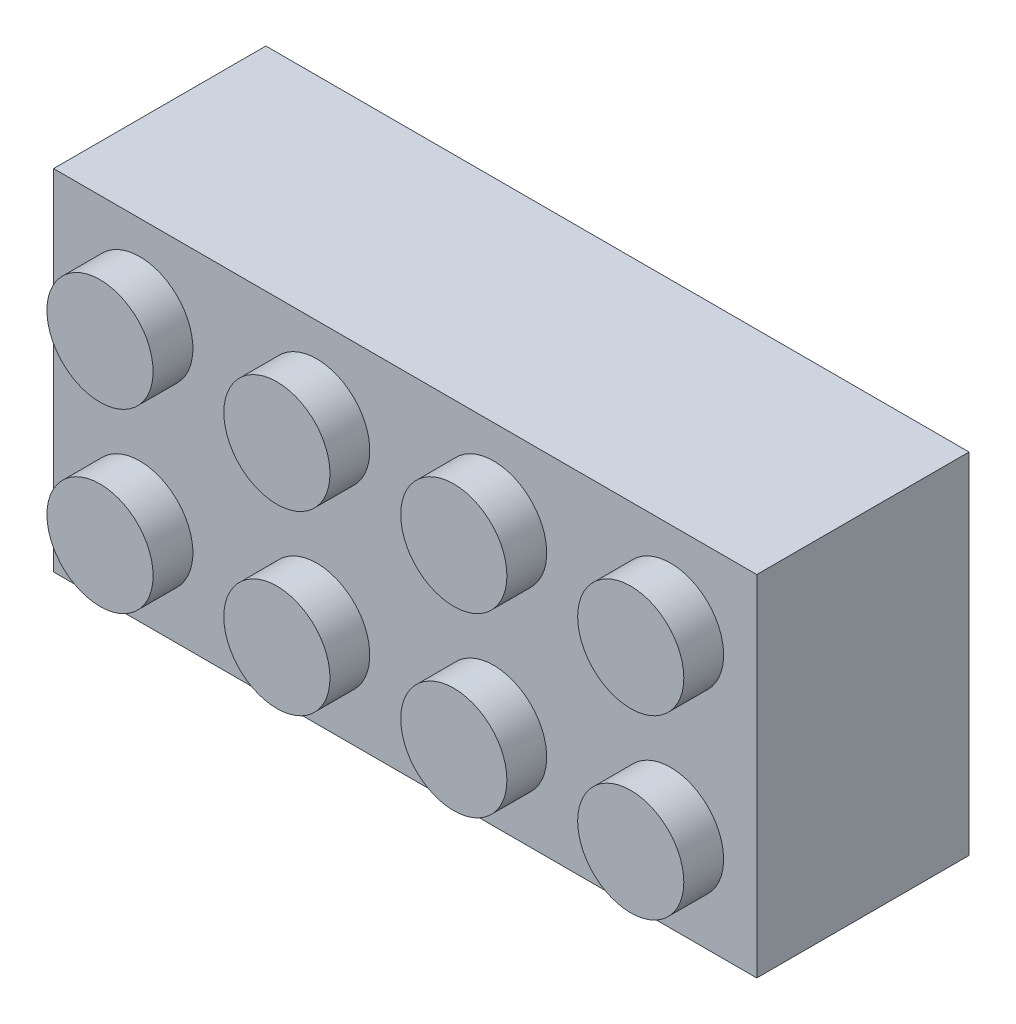
ISO-10303-21;
HEADER;
FILE_DESCRIPTION(('STEP AP214'),'2;1');
FILE_NAME('part.step','',(''),(''),'','','');
FILE_SCHEMA(('AUTOMOTIVE_DESIGN { 1 0 10303 214 1 1 1 1 }'));
ENDSEC;
DATA;
#1=APPLICATION_CONTEXT('core data for automotive mechanical design processes');
#2=APPLICATION_PROTOCOL_DEFINITION('international standard','automotive_design',2000,#1);
#3=PRODUCT_CONTEXT('',#1,'mechanical');
#4=PRODUCT('Part','Part','',(#3));
#5=PRODUCT_RELATED_PRODUCT_CATEGORY('part','',(#4));
#6=PRODUCT_DEFINITION_FORMATION('','',#4);
#7=PRODUCT_DEFINITION_CONTEXT('part definition',#1,'design');
#8=PRODUCT_DEFINITION('design','',#6,#7);
#9=PRODUCT_DEFINITION_SHAPE('','',#8);
#10=(LENGTH_UNIT() NAMED_UNIT(*) SI_UNIT(.MILLI.,.METRE.));
#11=(NAMED_UNIT(*) PLANE_ANGLE_UNIT() SI_UNIT($,.RADIAN.));
#12=(NAMED_UNIT(*) SI_UNIT($,.STERADIAN.) SOLID_ANGLE_UNIT());
#13=UNCERTAINTY_MEASURE_WITH_UNIT(LENGTH_MEASURE(1.E-05),#10,'distance_accuracy_value','');
#14=(GEOMETRIC_REPRESENTATION_CONTEXT(3) GLOBAL_UNCERTAINTY_ASSIGNED_CONTEXT((#13)) GLOBAL_UNIT_ASSIGNED_CONTEXT((#10,
#11,#12)) REPRESENTATION_CONTEXT('',''));
#15=CARTESIAN_POINT('',(0.,0.,0.));
#16=DIRECTION('',(0.,0.,1.));
#17=DIRECTION('',(1.,0.,0.));
#18=AXIS2_PLACEMENT_3D('',#15,#16,#17);
#19=CARTESIAN_POINT('',(31.8,0.,9.6));
#20=DIRECTION('',(0.,1.,0.));
#21=DIRECTION('',(0.,0.,1.));
#22=AXIS2_PLACEMENT_3D('',#19,#20,#21);
#23=PLANE('',#22);
#24=DIRECTION('',(1.,0.,0.));
#25=VECTOR('',#24,1.);
#26=CARTESIAN_POINT('',(31.8,0.,0.));
#27=LINE('',#26,#25);
#28=CARTESIAN_POINT('',(0.,0.,0.));
#29=VERTEX_POINT('',#28);
#30=CARTESIAN_POINT('',(31.8,0.,0.));
#31=VERTEX_POINT('',#30);
#32=EDGE_CURVE('E186',#29,#31,#27,.T.);
#33=ORIENTED_EDGE('',*,*,#32,.T.);
#34=DIRECTION('',(0.,0.,-1.));
#35=VECTOR('',#34,1.);
#36=CARTESIAN_POINT('',(31.8,0.,9.6));
#37=LINE('',#36,#35);
#38=CARTESIAN_POINT('',(31.8,0.,9.6));
#39=VERTEX_POINT('',#38);
#40=EDGE_CURVE('E213',#39,#31,#37,.T.);
#41=ORIENTED_EDGE('',*,*,#40,.F.);
#42=DIRECTION('',(1.,0.,0.));
#43=VECTOR('',#42,1.);
#44=CARTESIAN_POINT('',(31.8,0.,9.6));
#45=LINE('',#44,#43);
#46=CARTESIAN_POINT('',(0.,0.,9.6));
#47=VERTEX_POINT('',#46);
#48=EDGE_CURVE('E190',#47,#39,#45,.T.);
#49=ORIENTED_EDGE('',*,*,#48,.F.);
#50=DIRECTION('',(0.,0.,-1.));
#51=VECTOR('',#50,1.);
#52=CARTESIAN_POINT('',(0.,0.,9.6));
#53=LINE('',#52,#51);
#54=EDGE_CURVE('E197',#47,#29,#53,.T.);
#55=ORIENTED_EDGE('',*,*,#54,.T.);
#56=EDGE_LOOP('',(#33,#41,#49,#55));
#57=FACE_BOUND('',#56,.T.);
#58=ADVANCED_FACE('F42',(#57),#23,.F.);
#59=CARTESIAN_POINT('',(31.8,15.8,9.6));
#60=DIRECTION('',(-1.,0.,0.));
#61=DIRECTION('',(0.,0.,1.));
#62=AXIS2_PLACEMENT_3D('',#59,#60,#61);
#63=PLANE('',#62);
#64=DIRECTION('',(0.,1.,0.));
#65=VECTOR('',#64,1.);
#66=CARTESIAN_POINT('',(31.8,15.8,0.));
#67=LINE('',#66,#65);
#68=CARTESIAN_POINT('',(31.8,15.8,0.));
#69=VERTEX_POINT('',#68);
#70=EDGE_CURVE('E199',#31,#69,#67,.T.);
#71=ORIENTED_EDGE('',*,*,#70,.T.);
#72=DIRECTION('',(0.,0.,-1.));
#73=VECTOR('',#72,1.);
#74=CARTESIAN_POINT('',(31.8,15.8,9.6));
#75=LINE('',#74,#73);
#76=CARTESIAN_POINT('',(31.8,15.8,9.6));
#77=VERTEX_POINT('',#76);
#78=EDGE_CURVE('E209',#77,#69,#75,.T.);
#79=ORIENTED_EDGE('',*,*,#78,.F.);
#80=DIRECTION('',(0.,1.,0.));
#81=VECTOR('',#80,1.);
#82=CARTESIAN_POINT('',(31.8,15.8,9.6));
#83=LINE('',#82,#81);
#84=EDGE_CURVE('E189',#39,#77,#83,.T.);
#85=ORIENTED_EDGE('',*,*,#84,.F.);
#86=ORIENTED_EDGE('',*,*,#40,.T.);
#87=EDGE_LOOP('',(#71,#79,#85,#86));
#88=FACE_BOUND('',#87,.T.);
#89=ADVANCED_FACE('F264',(#88),#63,.F.);
#90=CARTESIAN_POINT('',(0.,15.8,9.6));
#91=DIRECTION('',(0.,-1.,0.));
#92=DIRECTION('',(0.,0.,-1.));
#93=AXIS2_PLACEMENT_3D('',#90,#91,#92);
#94=PLANE('',#93);
#95=DIRECTION('',(-1.,0.,0.));
#96=VECTOR('',#95,1.);
#97=CARTESIAN_POINT('',(0.,15.8,0.));
#98=LINE('',#97,#96);
#99=CARTESIAN_POINT('',(0.,15.8,0.));
#100=VERTEX_POINT('',#99);
#101=EDGE_CURVE('E205',#69,#100,#98,.T.);
#102=ORIENTED_EDGE('',*,*,#101,.T.);
#103=DIRECTION('',(0.,0.,-1.));
#104=VECTOR('',#103,1.);
#105=CARTESIAN_POINT('',(0.,15.8,9.6));
#106=LINE('',#105,#104);
#107=CARTESIAN_POINT('',(0.,15.8,9.6));
#108=VERTEX_POINT('',#107);
#109=EDGE_CURVE('E210',#108,#100,#106,.T.);
#110=ORIENTED_EDGE('',*,*,#109,.F.);
#111=DIRECTION('',(-1.,0.,0.));
#112=VECTOR('',#111,1.);
#113=CARTESIAN_POINT('',(0.,15.8,9.6));
#114=LINE('',#113,#112);
#115=EDGE_CURVE('E195',#77,#108,#114,.T.);
#116=ORIENTED_EDGE('',*,*,#115,.F.);
#117=ORIENTED_EDGE('',*,*,#78,.T.);
#118=EDGE_LOOP('',(#102,#110,#116,#117));
#119=FACE_BOUND('',#118,.T.);
#120=ADVANCED_FACE('F269',(#119),#94,.F.);
#121=CARTESIAN_POINT('',(0.,0.,9.6));
#122=DIRECTION('',(1.,0.,0.));
#123=DIRECTION('',(0.,0.,-1.));
#124=AXIS2_PLACEMENT_3D('',#121,#122,#123);
#125=PLANE('',#124);
#126=DIRECTION('',(0.,-1.,0.));
#127=VECTOR('',#126,1.);
#128=CARTESIAN_POINT('',(0.,0.,0.));
#129=LINE('',#128,#127);
#130=EDGE_CURVE('E192',#100,#29,#129,.T.);
#131=ORIENTED_EDGE('',*,*,#130,.T.);
#132=ORIENTED_EDGE('',*,*,#54,.F.);
#133=DIRECTION('',(0.,-1.,0.));
#134=VECTOR('',#133,1.);
#135=CARTESIAN_POINT('',(0.,0.,9.6));
#136=LINE('',#135,#134);
#137=EDGE_CURVE('E193',#108,#47,#136,.T.);
#138=ORIENTED_EDGE('',*,*,#137,.F.);
#139=ORIENTED_EDGE('',*,*,#109,.T.);
#140=EDGE_LOOP('',(#131,#132,#138,#139));
#141=FACE_BOUND('',#140,.T.);
#142=ADVANCED_FACE('F245',(#141),#125,.F.);
#143=CARTESIAN_POINT('',(0.,0.,9.6));
#144=DIRECTION('',(0.,0.,-1.));
#145=DIRECTION('',(-1.,0.,0.));
#146=AXIS2_PLACEMENT_3D('',#143,#144,#145);
#147=PLANE('',#146);
#148=CARTESIAN_POINT('',(27.9,3.9,9.6));
#149=DIRECTION('',(0.,0.,-1.));
#150=DIRECTION('',(-1.,0.,0.));
#151=AXIS2_PLACEMENT_3D('',#148,#149,#150);
#152=CIRCLE('',#151,2.4);
#153=CARTESIAN_POINT('',(25.5,3.9,9.6));
#154=VERTEX_POINT('',#153);
#155=EDGE_CURVE('E11',#154,#154,#152,.F.);
#156=ORIENTED_EDGE('',*,*,#155,.F.);
#157=EDGE_LOOP('',(#156));
#158=FACE_BOUND('',#157,.T.);
#159=CARTESIAN_POINT('',(19.9,3.9,9.6));
#160=DIRECTION('',(0.,0.,-1.));
#161=DIRECTION('',(-1.,0.,0.));
#162=AXIS2_PLACEMENT_3D('',#159,#160,#161);
#163=CIRCLE('',#162,2.4);
#164=CARTESIAN_POINT('',(17.5,3.9,9.6));
#165=VERTEX_POINT('',#164);
#166=EDGE_CURVE('E55',#165,#165,#163,.F.);
#167=ORIENTED_EDGE('',*,*,#166,.F.);
#168=EDGE_LOOP('',(#167));
#169=FACE_BOUND('',#168,.T.);
#170=CARTESIAN_POINT('',(11.9,3.9,9.6));
#171=DIRECTION('',(0.,0.,-1.));
#172=DIRECTION('',(-1.,0.,0.));
#173=AXIS2_PLACEMENT_3D('',#170,#171,#172);
#174=CIRCLE('',#173,2.4);
#175=CARTESIAN_POINT('',(9.5,3.9,9.6));
#176=VERTEX_POINT('',#175);
#177=EDGE_CURVE('E232',#176,#176,#174,.F.);
#178=ORIENTED_EDGE('',*,*,#177,.F.);
#179=EDGE_LOOP('',(#178));
#180=FACE_BOUND('',#179,.T.);
#181=CARTESIAN_POINT('',(27.9,11.9,9.6));
#182=DIRECTION('',(0.,0.,-1.));
#183=DIRECTION('',(-1.,0.,0.));
#184=AXIS2_PLACEMENT_3D('',#181,#182,#183);
#185=CIRCLE('',#184,2.4);
#186=CARTESIAN_POINT('',(25.5,11.9,9.6));
#187=VERTEX_POINT('',#186);
#188=EDGE_CURVE('E227',#187,#187,#185,.F.);
#189=ORIENTED_EDGE('',*,*,#188,.F.);
#190=EDGE_LOOP('',(#189));
#191=FACE_BOUND('',#190,.T.);
#192=CARTESIAN_POINT('',(19.9,11.9,9.6));
#193=DIRECTION('',(0.,0.,-1.));
#194=DIRECTION('',(-1.,0.,0.));
#195=AXIS2_PLACEMENT_3D('',#192,#193,#194);
#196=CIRCLE('',#195,2.4);
#197=CARTESIAN_POINT('',(17.5,11.9,9.6));
#198=VERTEX_POINT('',#197);
#199=EDGE_CURVE('E223',#198,#198,#196,.F.);
#200=ORIENTED_EDGE('',*,*,#199,.F.);
#201=EDGE_LOOP('',(#200));
#202=FACE_BOUND('',#201,.T.);
#203=CARTESIAN_POINT('',(11.9,11.9,9.6));
#204=DIRECTION('',(0.,0.,-1.));
#205=DIRECTION('',(-1.,0.,0.));
#206=AXIS2_PLACEMENT_3D('',#203,#204,#205);
#207=CIRCLE('',#206,2.4);
#208=CARTESIAN_POINT('',(9.5,11.9,9.6));
#209=VERTEX_POINT('',#208);
#210=EDGE_CURVE('E225',#209,#209,#207,.F.);
#211=ORIENTED_EDGE('',*,*,#210,.F.);
#212=EDGE_LOOP('',(#211));
#213=FACE_BOUND('',#212,.T.);
#214=CARTESIAN_POINT('',(3.9,3.9,9.6));
#215=DIRECTION('',(0.,0.,-1.));
#216=DIRECTION('',(-1.,0.,0.));
#217=AXIS2_PLACEMENT_3D('',#214,#215,#216);
#218=CIRCLE('',#217,2.4);
#219=CARTESIAN_POINT('',(1.5,3.9,9.6));
#220=VERTEX_POINT('',#219);
#221=EDGE_CURVE('E218',#220,#220,#218,.F.);
#222=ORIENTED_EDGE('',*,*,#221,.F.);
#223=EDGE_LOOP('',(#222));
#224=FACE_BOUND('',#223,.T.);
#225=CARTESIAN_POINT('',(3.9,11.9,9.6));
#226=DIRECTION('',(0.,0.,-1.));
#227=DIRECTION('',(-1.,0.,0.));
#228=AXIS2_PLACEMENT_3D('',#225,#226,#227);
#229=CIRCLE('',#228,2.4);
#230=CARTESIAN_POINT('',(1.5,11.9,9.6));
#231=VERTEX_POINT('',#230);
#232=EDGE_CURVE('E216',#231,#231,#229,.F.);
#233=ORIENTED_EDGE('',*,*,#232,.F.);
#234=EDGE_LOOP('',(#233));
#235=FACE_BOUND('',#234,.T.);
#236=ORIENTED_EDGE('',*,*,#48,.T.);
#237=ORIENTED_EDGE('',*,*,#84,.T.);
#238=ORIENTED_EDGE('',*,*,#115,.T.);
#239=ORIENTED_EDGE('',*,*,#137,.T.);
#240=EDGE_LOOP('',(#236,#237,#238,#239));
#241=FACE_BOUND('',#240,.T.);
#242=ADVANCED_FACE('F236',(#158,#169,#180,#191,#202,#213,#224,#235,#241),#147,.F.);
#243=CARTESIAN_POINT('',(0.,0.,0.));
#244=DIRECTION('',(0.,0.,-1.));
#245=DIRECTION('',(-1.,0.,0.));
#246=AXIS2_PLACEMENT_3D('',#243,#244,#245);
#247=PLANE('',#246);
#248=ORIENTED_EDGE('',*,*,#32,.F.);
#249=ORIENTED_EDGE('',*,*,#130,.F.);
#250=ORIENTED_EDGE('',*,*,#101,.F.);
#251=ORIENTED_EDGE('',*,*,#70,.F.);
#252=EDGE_LOOP('',(#248,#249,#250,#251));
#253=FACE_BOUND('',#252,.T.);
#254=ADVANCED_FACE('F241',(#253),#247,.T.);
#255=CARTESIAN_POINT('',(3.9,11.9,11.4));
#256=DIRECTION('',(0.,0.,-1.));
#257=DIRECTION('',(-1.,0.,0.));
#258=AXIS2_PLACEMENT_3D('',#255,#256,#257);
#259=CYLINDRICAL_SURFACE('',#258,2.4);
#260=CARTESIAN_POINT('',(3.9,11.9,11.4));
#261=DIRECTION('',(0.,0.,1.));
#262=DIRECTION('',(1.,0.,0.));
#263=AXIS2_PLACEMENT_3D('',#260,#261,#262);
#264=CIRCLE('',#263,2.4);
#265=CARTESIAN_POINT('',(6.3,11.9,11.4));
#266=VERTEX_POINT('',#265);
#267=EDGE_CURVE('E181',#266,#266,#264,.T.);
#268=ORIENTED_EDGE('',*,*,#267,.F.);
#269=EDGE_LOOP('',(#268));
#270=FACE_BOUND('',#269,.T.);
#271=ORIENTED_EDGE('',*,*,#232,.T.);
#272=EDGE_LOOP('',(#271));
#273=FACE_BOUND('',#272,.T.);
#274=ADVANCED_FACE('F274',(#270,#273),#259,.T.);
#275=CARTESIAN_POINT('',(3.9,11.9,11.4));
#276=DIRECTION('',(0.,0.,1.));
#277=DIRECTION('',(1.,0.,0.));
#278=AXIS2_PLACEMENT_3D('',#275,#276,#277);
#279=PLANE('',#278);
#280=ORIENTED_EDGE('',*,*,#267,.T.);
#281=EDGE_LOOP('',(#280));
#282=FACE_BOUND('',#281,.T.);
#283=ADVANCED_FACE('F281',(#282),#279,.T.);
#284=CARTESIAN_POINT('',(3.9,3.9,11.4));
#285=DIRECTION('',(0.,0.,-1.));
#286=DIRECTION('',(-1.,0.,0.));
#287=AXIS2_PLACEMENT_3D('',#284,#285,#286);
#288=CYLINDRICAL_SURFACE('',#287,2.4);
#289=CARTESIAN_POINT('',(3.9,3.9,11.4));
#290=DIRECTION('',(0.,0.,1.));
#291=DIRECTION('',(1.,0.,0.));
#292=AXIS2_PLACEMENT_3D('',#289,#290,#291);
#293=CIRCLE('',#292,2.4);
#294=CARTESIAN_POINT('',(6.3,3.9,11.4));
#295=VERTEX_POINT('',#294);
#296=EDGE_CURVE('E178',#295,#295,#293,.T.);
#297=ORIENTED_EDGE('',*,*,#296,.F.);
#298=EDGE_LOOP('',(#297));
#299=FACE_BOUND('',#298,.T.);
#300=ORIENTED_EDGE('',*,*,#221,.T.);
#301=EDGE_LOOP('',(#300));
#302=FACE_BOUND('',#301,.T.);
#303=ADVANCED_FACE('F332',(#299,#302),#288,.T.);
#304=CARTESIAN_POINT('',(3.9,3.9,11.4));
#305=DIRECTION('',(0.,0.,1.));
#306=DIRECTION('',(1.,0.,0.));
#307=AXIS2_PLACEMENT_3D('',#304,#305,#306);
#308=PLANE('',#307);
#309=ORIENTED_EDGE('',*,*,#296,.T.);
#310=EDGE_LOOP('',(#309));
#311=FACE_BOUND('',#310,.T.);
#312=ADVANCED_FACE('F342',(#311),#308,.T.);
#313=CARTESIAN_POINT('',(11.9,11.9,11.4));
#314=DIRECTION('',(0.,0.,-1.));
#315=DIRECTION('',(-1.,0.,0.));
#316=AXIS2_PLACEMENT_3D('',#313,#314,#315);
#317=CYLINDRICAL_SURFACE('',#316,2.4);
#318=CARTESIAN_POINT('',(11.9,11.9,11.4));
#319=DIRECTION('',(0.,0.,1.));
#320=DIRECTION('',(1.,0.,0.));
#321=AXIS2_PLACEMENT_3D('',#318,#319,#320);
#322=CIRCLE('',#321,2.4);
#323=CARTESIAN_POINT('',(14.3,11.9,11.4));
#324=VERTEX_POINT('',#323);
#325=EDGE_CURVE('E179',#324,#324,#322,.T.);
#326=ORIENTED_EDGE('',*,*,#325,.F.);
#327=EDGE_LOOP('',(#326));
#328=FACE_BOUND('',#327,.T.);
#329=ORIENTED_EDGE('',*,*,#210,.T.);
#330=EDGE_LOOP('',(#329));
#331=FACE_BOUND('',#330,.T.);
#332=ADVANCED_FACE('F351',(#328,#331),#317,.T.);
#333=CARTESIAN_POINT('',(11.9,11.9,11.4));
#334=DIRECTION('',(0.,0.,1.));
#335=DIRECTION('',(1.,0.,0.));
#336=AXIS2_PLACEMENT_3D('',#333,#334,#335);
#337=PLANE('',#336);
#338=ORIENTED_EDGE('',*,*,#325,.T.);
#339=EDGE_LOOP('',(#338));
#340=FACE_BOUND('',#339,.T.);
#341=ADVANCED_FACE('F363',(#340),#337,.T.);
#342=CARTESIAN_POINT('',(19.9,11.9,11.4));
#343=DIRECTION('',(0.,0.,-1.));
#344=DIRECTION('',(-1.,0.,0.));
#345=AXIS2_PLACEMENT_3D('',#342,#343,#344);
#346=CYLINDRICAL_SURFACE('',#345,2.4);
#347=CARTESIAN_POINT('',(19.9,11.9,11.4));
#348=DIRECTION('',(0.,0.,1.));
#349=DIRECTION('',(1.,0.,0.));
#350=AXIS2_PLACEMENT_3D('',#347,#348,#349);
#351=CIRCLE('',#350,2.4);
#352=CARTESIAN_POINT('',(22.3,11.9,11.4));
#353=VERTEX_POINT('',#352);
#354=EDGE_CURVE('E173',#353,#353,#351,.T.);
#355=ORIENTED_EDGE('',*,*,#354,.F.);
#356=EDGE_LOOP('',(#355));
#357=FACE_BOUND('',#356,.T.);
#358=ORIENTED_EDGE('',*,*,#199,.T.);
#359=EDGE_LOOP('',(#358));
#360=FACE_BOUND('',#359,.T.);
#361=ADVANCED_FACE('F371',(#357,#360),#346,.T.);
#362=CARTESIAN_POINT('',(19.9,11.9,11.4));
#363=DIRECTION('',(0.,0.,1.));
#364=DIRECTION('',(1.,0.,0.));
#365=AXIS2_PLACEMENT_3D('',#362,#363,#364);
#366=PLANE('',#365);
#367=ORIENTED_EDGE('',*,*,#354,.T.);
#368=EDGE_LOOP('',(#367));
#369=FACE_BOUND('',#368,.T.);
#370=ADVANCED_FACE('F381',(#369),#366,.T.);
#371=CARTESIAN_POINT('',(27.9,11.9,11.4));
#372=DIRECTION('',(0.,0.,-1.));
#373=DIRECTION('',(-1.,0.,0.));
#374=AXIS2_PLACEMENT_3D('',#371,#372,#373);
#375=CYLINDRICAL_SURFACE('',#374,2.4);
#376=CARTESIAN_POINT('',(27.9,11.9,11.4));
#377=DIRECTION('',(0.,0.,1.));
#378=DIRECTION('',(1.,0.,0.));
#379=AXIS2_PLACEMENT_3D('',#376,#377,#378);
#380=CIRCLE('',#379,2.4);
#381=CARTESIAN_POINT('',(30.3,11.9,11.4));
#382=VERTEX_POINT('',#381);
#383=EDGE_CURVE('E171',#382,#382,#380,.T.);
#384=ORIENTED_EDGE('',*,*,#383,.F.);
#385=EDGE_LOOP('',(#384));
#386=FACE_BOUND('',#385,.T.);
#387=ORIENTED_EDGE('',*,*,#188,.T.);
#388=EDGE_LOOP('',(#387));
#389=FACE_BOUND('',#388,.T.);
#390=ADVANCED_FACE('F391',(#386,#389),#375,.T.);
#391=CARTESIAN_POINT('',(27.9,11.9,11.4));
#392=DIRECTION('',(0.,0.,1.));
#393=DIRECTION('',(1.,0.,0.));
#394=AXIS2_PLACEMENT_3D('',#391,#392,#393);
#395=PLANE('',#394);
#396=ORIENTED_EDGE('',*,*,#383,.T.);
#397=EDGE_LOOP('',(#396));
#398=FACE_BOUND('',#397,.T.);
#399=ADVANCED_FACE('F402',(#398),#395,.T.);
#400=CARTESIAN_POINT('',(11.9,3.9,11.4));
#401=DIRECTION('',(0.,0.,-1.));
#402=DIRECTION('',(-1.,0.,0.));
#403=AXIS2_PLACEMENT_3D('',#400,#401,#402);
#404=CYLINDRICAL_SURFACE('',#403,2.4);
#405=CARTESIAN_POINT('',(11.9,3.9,11.4));
#406=DIRECTION('',(0.,0.,1.));
#407=DIRECTION('',(1.,0.,0.));
#408=AXIS2_PLACEMENT_3D('',#405,#406,#407);
#409=CIRCLE('',#408,2.4);
#410=CARTESIAN_POINT('',(14.3,3.9,11.4));
#411=VERTEX_POINT('',#410);
#412=EDGE_CURVE('E169',#411,#411,#409,.T.);
#413=ORIENTED_EDGE('',*,*,#412,.F.);
#414=EDGE_LOOP('',(#413));
#415=FACE_BOUND('',#414,.T.);
#416=ORIENTED_EDGE('',*,*,#177,.T.);
#417=EDGE_LOOP('',(#416));
#418=FACE_BOUND('',#417,.T.);
#419=ADVANCED_FACE('F412',(#415,#418),#404,.T.);
#420=CARTESIAN_POINT('',(11.9,3.9,11.4));
#421=DIRECTION('',(0.,0.,1.));
#422=DIRECTION('',(1.,0.,0.));
#423=AXIS2_PLACEMENT_3D('',#420,#421,#422);
#424=PLANE('',#423);
#425=ORIENTED_EDGE('',*,*,#412,.T.);
#426=EDGE_LOOP('',(#425));
#427=FACE_BOUND('',#426,.T.);
#428=ADVANCED_FACE('F423',(#427),#424,.T.);
#429=CARTESIAN_POINT('',(19.9,3.9,11.4));
#430=DIRECTION('',(0.,0.,-1.));
#431=DIRECTION('',(-1.,0.,0.));
#432=AXIS2_PLACEMENT_3D('',#429,#430,#431);
#433=CYLINDRICAL_SURFACE('',#432,2.4);
#434=CARTESIAN_POINT('',(19.9,3.9,11.4));
#435=DIRECTION('',(0.,0.,1.));
#436=DIRECTION('',(1.,0.,0.));
#437=AXIS2_PLACEMENT_3D('',#434,#435,#436);
#438=CIRCLE('',#437,2.4);
#439=CARTESIAN_POINT('',(22.3,3.9,11.4));
#440=VERTEX_POINT('',#439);
#441=EDGE_CURVE('E163',#440,#440,#438,.T.);
#442=ORIENTED_EDGE('',*,*,#441,.F.);
#443=EDGE_LOOP('',(#442));
#444=FACE_BOUND('',#443,.T.);
#445=ORIENTED_EDGE('',*,*,#166,.T.);
#446=EDGE_LOOP('',(#445));
#447=FACE_BOUND('',#446,.T.);
#448=ADVANCED_FACE('F237',(#444,#447),#433,.T.);
#449=CARTESIAN_POINT('',(19.9,3.9,11.4));
#450=DIRECTION('',(0.,0.,1.));
#451=DIRECTION('',(1.,0.,0.));
#452=AXIS2_PLACEMENT_3D('',#449,#450,#451);
#453=PLANE('',#452);
#454=ORIENTED_EDGE('',*,*,#441,.T.);
#455=EDGE_LOOP('',(#454));
#456=FACE_BOUND('',#455,.T.);
#457=ADVANCED_FACE('F439',(#456),#453,.T.);
#458=CARTESIAN_POINT('',(27.9,3.9,11.4));
#459=DIRECTION('',(0.,0.,-1.));
#460=DIRECTION('',(-1.,0.,0.));
#461=AXIS2_PLACEMENT_3D('',#458,#459,#460);
#462=CYLINDRICAL_SURFACE('',#461,2.4);
#463=CARTESIAN_POINT('',(27.9,3.9,11.4));
#464=DIRECTION('',(0.,0.,1.));
#465=DIRECTION('',(1.,0.,0.));
#466=AXIS2_PLACEMENT_3D('',#463,#464,#465);
#467=CIRCLE('',#466,2.4);
#468=CARTESIAN_POINT('',(30.3,3.9,11.4));
#469=VERTEX_POINT('',#468);
#470=EDGE_CURVE('E161',#469,#469,#467,.T.);
#471=ORIENTED_EDGE('',*,*,#470,.F.);
#472=EDGE_LOOP('',(#471));
#473=FACE_BOUND('',#472,.T.);
#474=ORIENTED_EDGE('',*,*,#155,.T.);
#475=EDGE_LOOP('',(#474));
#476=FACE_BOUND('',#475,.T.);
#477=ADVANCED_FACE('F449',(#473,#476),#462,.T.);
#478=CARTESIAN_POINT('',(27.9,3.9,11.4));
#479=DIRECTION('',(0.,0.,1.));
#480=DIRECTION('',(1.,0.,0.));
#481=AXIS2_PLACEMENT_3D('',#478,#479,#480);
#482=PLANE('',#481);
#483=ORIENTED_EDGE('',*,*,#470,.T.);
#484=EDGE_LOOP('',(#483));
#485=FACE_BOUND('',#484,.T.);
#486=ADVANCED_FACE('F458',(#485),#482,.T.);
#487=CLOSED_SHELL('',(#58,#89,#120,#142,#242,#254,#274,#283,#303,#312,#332,#341,#361,#370,#390,
#399,#419,#428,#448,#457,#477,#486));
#488=CARTESIAN_POINT('',(0.,15.,0.));
#489=DIRECTION('',(0.,-1.,0.));
#490=DIRECTION('',(0.,0.,-1.));
#491=AXIS2_PLACEMENT_3D('',#488,#489,#490);
#492=PLANE('',#491);
#493=DIRECTION('',(0.,0.,1.));
#494=VECTOR('',#493,1.);
#495=CARTESIAN_POINT('',(16.3,15.,0.));
#496=LINE('',#495,#494);
#497=CARTESIAN_POINT('',(16.3,15.,2.5));
#498=VERTEX_POINT('',#497);
#499=CARTESIAN_POINT('',(16.3,15.,8.8));
#500=VERTEX_POINT('',#499);
#501=EDGE_CURVE('E691',#498,#500,#496,.T.);
#502=ORIENTED_EDGE('',*,*,#501,.F.);
#503=DIRECTION('',(1.,0.,0.));
#504=VECTOR('',#503,1.);
#505=CARTESIAN_POINT('',(0.,15.,2.5));
#506=LINE('',#505,#504);
#507=CARTESIAN_POINT('',(30.6,15.,2.5));
#508=VERTEX_POINT('',#507);
#509=EDGE_CURVE('E147',#498,#508,#506,.T.);
#510=ORIENTED_EDGE('',*,*,#509,.T.);
#511=DIRECTION('',(0.,0.,1.));
#512=VECTOR('',#511,1.);
#513=CARTESIAN_POINT('',(30.6,15.,0.));
#514=LINE('',#513,#512);
#515=CARTESIAN_POINT('',(30.6,15.,8.8));
#516=VERTEX_POINT('',#515);
#517=EDGE_CURVE('E160',#508,#516,#514,.T.);
#518=ORIENTED_EDGE('',*,*,#517,.T.);
#519=DIRECTION('',(-1.,0.,0.));
#520=VECTOR('',#519,1.);
#521=CARTESIAN_POINT('',(0.,15.,8.8));
#522=LINE('',#521,#520);
#523=EDGE_CURVE('E155',#516,#500,#522,.T.);
#524=ORIENTED_EDGE('',*,*,#523,.T.);
#525=EDGE_LOOP('',(#502,#510,#518,#524));
#526=FACE_BOUND('',#525,.T.);
#527=ADVANCED_FACE('F508',(#526),#492,.T.);
#528=CARTESIAN_POINT('',(0.,15.,2.5));
#529=DIRECTION('',(0.,0.,-1.));
#530=DIRECTION('',(-1.,0.,0.));
#531=AXIS2_PLACEMENT_3D('',#528,#529,#530);
#532=PLANE('',#531);
#533=DIRECTION('',(0.,-1.,0.));
#534=VECTOR('',#533,1.);
#535=CARTESIAN_POINT('',(16.3,15.,2.5));
#536=LINE('',#535,#534);
#537=CARTESIAN_POINT('',(16.3,1.,2.5));
#538=VERTEX_POINT('',#537);
#539=EDGE_CURVE('E142',#498,#538,#536,.T.);
#540=ORIENTED_EDGE('',*,*,#539,.T.);
#541=DIRECTION('',(1.,0.,0.));
#542=VECTOR('',#541,1.);
#543=CARTESIAN_POINT('',(30.6,1.,2.5));
#544=LINE('',#543,#542);
#545=CARTESIAN_POINT('',(30.6,1.,2.5));
#546=VERTEX_POINT('',#545);
#547=EDGE_CURVE('E128',#538,#546,#544,.T.);
#548=ORIENTED_EDGE('',*,*,#547,.T.);
#549=DIRECTION('',(0.,-1.,0.));
#550=VECTOR('',#549,1.);
#551=CARTESIAN_POINT('',(30.6,15.,2.5));
#552=LINE('',#551,#550);
#553=EDGE_CURVE('E151',#508,#546,#552,.T.);
#554=ORIENTED_EDGE('',*,*,#553,.F.);
#555=ORIENTED_EDGE('',*,*,#509,.F.);
#556=EDGE_LOOP('',(#540,#548,#554,#555));
#557=FACE_BOUND('',#556,.T.);
#558=ADVANCED_FACE('F146',(#557),#532,.F.);
#559=CARTESIAN_POINT('',(30.6,15.,0.));
#560=DIRECTION('',(1.,0.,0.));
#561=DIRECTION('',(0.,0.,-1.));
#562=AXIS2_PLACEMENT_3D('',#559,#560,#561);
#563=PLANE('',#562);
#564=ORIENTED_EDGE('',*,*,#553,.T.);
#565=DIRECTION('',(0.,0.,1.));
#566=VECTOR('',#565,1.);
#567=CARTESIAN_POINT('',(30.6,1.,8.8));
#568=LINE('',#567,#566);
#569=CARTESIAN_POINT('',(30.6,1.,8.8));
#570=VERTEX_POINT('',#569);
#571=EDGE_CURVE('E56',#546,#570,#568,.T.);
#572=ORIENTED_EDGE('',*,*,#571,.T.);
#573=DIRECTION('',(0.,-1.,0.));
#574=VECTOR('',#573,1.);
#575=CARTESIAN_POINT('',(30.6,15.,8.8));
#576=LINE('',#575,#574);
#577=EDGE_CURVE('E152',#516,#570,#576,.T.);
#578=ORIENTED_EDGE('',*,*,#577,.F.);
#579=ORIENTED_EDGE('',*,*,#517,.F.);
#580=EDGE_LOOP('',(#564,#572,#578,#579));
#581=FACE_BOUND('',#580,.T.);
#582=ADVANCED_FACE('F493',(#581),#563,.F.);
#583=CARTESIAN_POINT('',(0.,15.,8.8));
#584=DIRECTION('',(0.,0.,1.));
#585=DIRECTION('',(1.,0.,0.));
#586=AXIS2_PLACEMENT_3D('',#583,#584,#585);
#587=PLANE('',#586);
#588=ORIENTED_EDGE('',*,*,#577,.T.);
#589=DIRECTION('',(-1.,0.,0.));
#590=VECTOR('',#589,1.);
#591=CARTESIAN_POINT('',(16.3,1.,8.8));
#592=LINE('',#591,#590);
#593=CARTESIAN_POINT('',(16.3,1.,8.8));
#594=VERTEX_POINT('',#593);
#595=EDGE_CURVE('E701',#570,#594,#592,.T.);
#596=ORIENTED_EDGE('',*,*,#595,.T.);
#597=DIRECTION('',(0.,-1.,0.));
#598=VECTOR('',#597,1.);
#599=CARTESIAN_POINT('',(16.3,15.,8.8));
#600=LINE('',#599,#598);
#601=EDGE_CURVE('E144',#500,#594,#600,.T.);
#602=ORIENTED_EDGE('',*,*,#601,.F.);
#603=ORIENTED_EDGE('',*,*,#523,.F.);
#604=EDGE_LOOP('',(#588,#596,#602,#603));
#605=FACE_BOUND('',#604,.T.);
#606=ADVANCED_FACE('F484',(#605),#587,.F.);
#607=CARTESIAN_POINT('',(16.3,15.,0.));
#608=DIRECTION('',(1.,0.,0.));
#609=DIRECTION('',(0.,0.,-1.));
#610=AXIS2_PLACEMENT_3D('',#607,#608,#609);
#611=PLANE('',#610);
#612=DIRECTION('',(0.,0.,-1.));
#613=VECTOR('',#612,1.);
#614=CARTESIAN_POINT('',(16.3,1.,2.5));
#615=LINE('',#614,#613);
#616=EDGE_CURVE('E132',#594,#538,#615,.T.);
#617=ORIENTED_EDGE('',*,*,#616,.T.);
#618=ORIENTED_EDGE('',*,*,#539,.F.);
#619=ORIENTED_EDGE('',*,*,#501,.T.);
#620=ORIENTED_EDGE('',*,*,#601,.T.);
#621=EDGE_LOOP('',(#617,#618,#619,#620));
#622=FACE_BOUND('',#621,.T.);
#623=ADVANCED_FACE('F143',(#622),#611,.T.);
#624=CARTESIAN_POINT('',(0.,1.,0.));
#625=DIRECTION('',(0.,1.,0.));
#626=DIRECTION('',(0.,0.,1.));
#627=AXIS2_PLACEMENT_3D('',#624,#625,#626);
#628=PLANE('',#627);
#629=ORIENTED_EDGE('',*,*,#616,.F.);
#630=ORIENTED_EDGE('',*,*,#595,.F.);
#631=ORIENTED_EDGE('',*,*,#571,.F.);
#632=ORIENTED_EDGE('',*,*,#547,.F.);
#633=EDGE_LOOP('',(#629,#630,#631,#632));
#634=FACE_BOUND('',#633,.T.);
#635=ADVANCED_FACE('F135',(#634),#628,.T.);
#636=CLOSED_SHELL('',(#527,#558,#582,#606,#623,#635));
#637=CARTESIAN_POINT('',(0.,15.,0.));
#638=DIRECTION('',(0.,-1.,0.));
#639=DIRECTION('',(0.,0.,-1.));
#640=AXIS2_PLACEMENT_3D('',#637,#638,#639);
#641=PLANE('',#640);
#642=DIRECTION('',(0.,0.,-1.));
#643=VECTOR('',#642,1.);
#644=CARTESIAN_POINT('',(15.5,15.,0.));
#645=LINE('',#644,#643);
#646=CARTESIAN_POINT('',(15.5,15.,8.8));
#647=VERTEX_POINT('',#646);
#648=CARTESIAN_POINT('',(15.5,15.,2.5));
#649=VERTEX_POINT('',#648);
#650=EDGE_CURVE('E670',#647,#649,#645,.T.);
#651=ORIENTED_EDGE('',*,*,#650,.F.);
#652=DIRECTION('',(-1.,0.,0.));
#653=VECTOR('',#652,1.);
#654=CARTESIAN_POINT('',(0.,15.,8.8));
#655=LINE('',#654,#653);
#656=CARTESIAN_POINT('',(1.5,15.,8.8));
#657=VERTEX_POINT('',#656);
#658=EDGE_CURVE('E669',#647,#657,#655,.T.);
#659=ORIENTED_EDGE('',*,*,#658,.T.);
#660=DIRECTION('',(0.,0.,-1.));
#661=VECTOR('',#660,1.);
#662=CARTESIAN_POINT('',(1.5,15.,0.));
#663=LINE('',#662,#661);
#664=CARTESIAN_POINT('',(1.5,15.,2.5));
#665=VERTEX_POINT('',#664);
#666=EDGE_CURVE('E681',#657,#665,#663,.T.);
#667=ORIENTED_EDGE('',*,*,#666,.T.);
#668=DIRECTION('',(1.,0.,0.));
#669=VECTOR('',#668,1.);
#670=CARTESIAN_POINT('',(0.,15.,2.5));
#671=LINE('',#670,#669);
#672=EDGE_CURVE('E674',#665,#649,#671,.T.);
#673=ORIENTED_EDGE('',*,*,#672,.T.);
#674=EDGE_LOOP('',(#651,#659,#667,#673));
#675=FACE_BOUND('',#674,.T.);
#676=ADVANCED_FACE('F560',(#675),#641,.T.);
#677=CARTESIAN_POINT('',(0.,15.,8.8));
#678=DIRECTION('',(0.,0.,1.));
#679=DIRECTION('',(1.,0.,0.));
#680=AXIS2_PLACEMENT_3D('',#677,#678,#679);
#681=PLANE('',#680);
#682=DIRECTION('',(0.,-1.,0.));
#683=VECTOR('',#682,1.);
#684=CARTESIAN_POINT('',(15.5,15.,8.8));
#685=LINE('',#684,#683);
#686=CARTESIAN_POINT('',(15.5,1.,8.8));
#687=VERTEX_POINT('',#686);
#688=EDGE_CURVE('E680',#647,#687,#685,.T.);
#689=ORIENTED_EDGE('',*,*,#688,.T.);
#690=DIRECTION('',(-1.,0.,0.));
#691=VECTOR('',#690,1.);
#692=CARTESIAN_POINT('',(1.5,1.,8.8));
#693=LINE('',#692,#691);
#694=CARTESIAN_POINT('',(1.5,1.,8.8));
#695=VERTEX_POINT('',#694);
#696=EDGE_CURVE('E694',#687,#695,#693,.T.);
#697=ORIENTED_EDGE('',*,*,#696,.T.);
#698=DIRECTION('',(0.,-1.,0.));
#699=VECTOR('',#698,1.);
#700=CARTESIAN_POINT('',(1.5,15.,8.8));
#701=LINE('',#700,#699);
#702=EDGE_CURVE('E679',#657,#695,#701,.T.);
#703=ORIENTED_EDGE('',*,*,#702,.F.);
#704=ORIENTED_EDGE('',*,*,#658,.F.);
#705=EDGE_LOOP('',(#689,#697,#703,#704));
#706=FACE_BOUND('',#705,.T.);
#707=ADVANCED_FACE('F547',(#706),#681,.F.);
#708=CARTESIAN_POINT('',(1.5,15.,0.));
#709=DIRECTION('',(-1.,0.,0.));
#710=DIRECTION('',(0.,0.,1.));
#711=AXIS2_PLACEMENT_3D('',#708,#709,#710);
#712=PLANE('',#711);
#713=ORIENTED_EDGE('',*,*,#702,.T.);
#714=DIRECTION('',(0.,0.,-1.));
#715=VECTOR('',#714,1.);
#716=CARTESIAN_POINT('',(1.5,1.,2.5));
#717=LINE('',#716,#715);
#718=CARTESIAN_POINT('',(1.5,1.,2.5));
#719=VERTEX_POINT('',#718);
#720=EDGE_CURVE('E69',#695,#719,#717,.T.);
#721=ORIENTED_EDGE('',*,*,#720,.T.);
#722=DIRECTION('',(0.,-1.,0.));
#723=VECTOR('',#722,1.);
#724=CARTESIAN_POINT('',(1.5,15.,2.5));
#725=LINE('',#724,#723);
#726=EDGE_CURVE('E690',#665,#719,#725,.T.);
#727=ORIENTED_EDGE('',*,*,#726,.F.);
#728=ORIENTED_EDGE('',*,*,#666,.F.);
#729=EDGE_LOOP('',(#713,#721,#727,#728));
#730=FACE_BOUND('',#729,.T.);
#731=ADVANCED_FACE('F537',(#730),#712,.F.);
#732=CARTESIAN_POINT('',(0.,15.,2.5));
#733=DIRECTION('',(0.,0.,-1.));
#734=DIRECTION('',(-1.,0.,0.));
#735=AXIS2_PLACEMENT_3D('',#732,#733,#734);
#736=PLANE('',#735);
#737=ORIENTED_EDGE('',*,*,#726,.T.);
#738=DIRECTION('',(1.,0.,0.));
#739=VECTOR('',#738,1.);
#740=CARTESIAN_POINT('',(15.5,1.,2.5));
#741=LINE('',#740,#739);
#742=CARTESIAN_POINT('',(15.5,1.,2.5));
#743=VERTEX_POINT('',#742);
#744=EDGE_CURVE('E710',#719,#743,#741,.T.);
#745=ORIENTED_EDGE('',*,*,#744,.T.);
#746=DIRECTION('',(0.,-1.,0.));
#747=VECTOR('',#746,1.);
#748=CARTESIAN_POINT('',(15.5,15.,2.5));
#749=LINE('',#748,#747);
#750=EDGE_CURVE('E164',#649,#743,#749,.T.);
#751=ORIENTED_EDGE('',*,*,#750,.F.);
#752=ORIENTED_EDGE('',*,*,#672,.F.);
#753=EDGE_LOOP('',(#737,#745,#751,#752));
#754=FACE_BOUND('',#753,.T.);
#755=ADVANCED_FACE('F526',(#754),#736,.F.);
#756=CARTESIAN_POINT('',(15.5,15.,0.));
#757=DIRECTION('',(-1.,0.,0.));
#758=DIRECTION('',(0.,0.,1.));
#759=AXIS2_PLACEMENT_3D('',#756,#757,#758);
#760=PLANE('',#759);
#761=DIRECTION('',(0.,0.,1.));
#762=VECTOR('',#761,1.);
#763=CARTESIAN_POINT('',(15.5,1.,8.8));
#764=LINE('',#763,#762);
#765=EDGE_CURVE('E709',#743,#687,#764,.T.);
#766=ORIENTED_EDGE('',*,*,#765,.T.);
#767=ORIENTED_EDGE('',*,*,#688,.F.);
#768=ORIENTED_EDGE('',*,*,#650,.T.);
#769=ORIENTED_EDGE('',*,*,#750,.T.);
#770=EDGE_LOOP('',(#766,#767,#768,#769));
#771=FACE_BOUND('',#770,.T.);
#772=ADVANCED_FACE('F525',(#771),#760,.T.);
#773=CARTESIAN_POINT('',(0.,1.,0.));
#774=DIRECTION('',(0.,1.,0.));
#775=DIRECTION('',(0.,0.,1.));
#776=AXIS2_PLACEMENT_3D('',#773,#774,#775);
#777=PLANE('',#776);
#778=ORIENTED_EDGE('',*,*,#720,.F.);
#779=ORIENTED_EDGE('',*,*,#696,.F.);
#780=ORIENTED_EDGE('',*,*,#765,.F.);
#781=ORIENTED_EDGE('',*,*,#744,.F.);
#782=EDGE_LOOP('',(#778,#779,#780,#781));
#783=FACE_BOUND('',#782,.T.);
#784=ADVANCED_FACE('F527',(#783),#777,.T.);
#785=CLOSED_SHELL('',(#676,#707,#731,#755,#772,#784));
#786=ORIENTED_CLOSED_SHELL('',*,#636,.T.);
#787=ORIENTED_CLOSED_SHELL('',*,#785,.T.);
#788=BREP_WITH_VOIDS('B2',#487,(#786,#787));
#789=ADVANCED_BREP_SHAPE_REPRESENTATION('',(#18,#788),#14);
#790=SHAPE_DEFINITION_REPRESENTATION(#9,#789);
ENDSEC;
END-ISO-10303-21;
